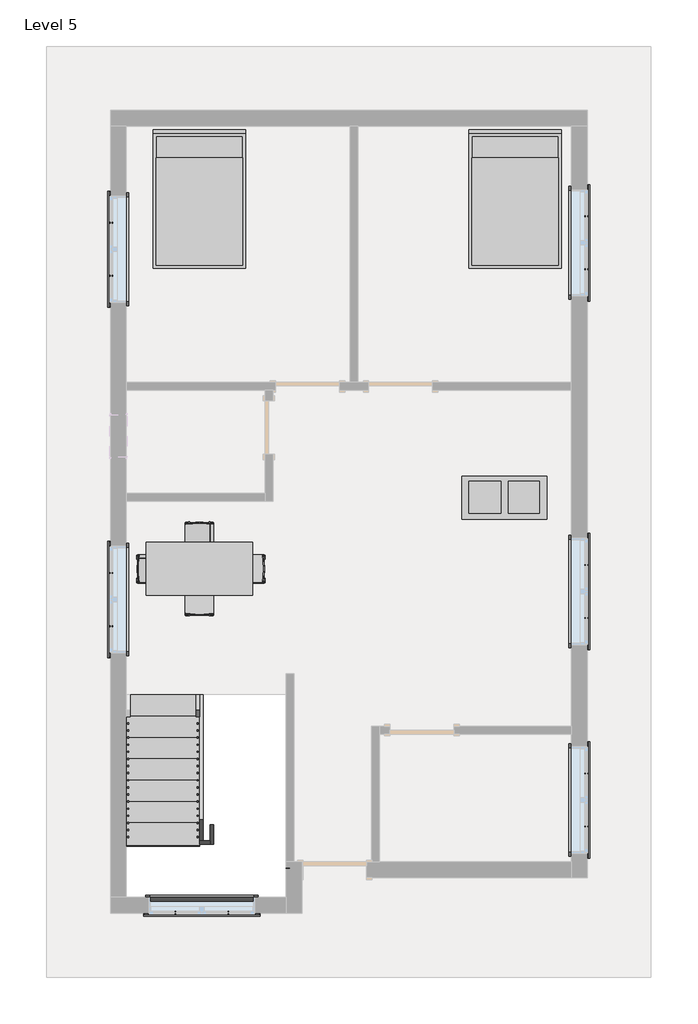
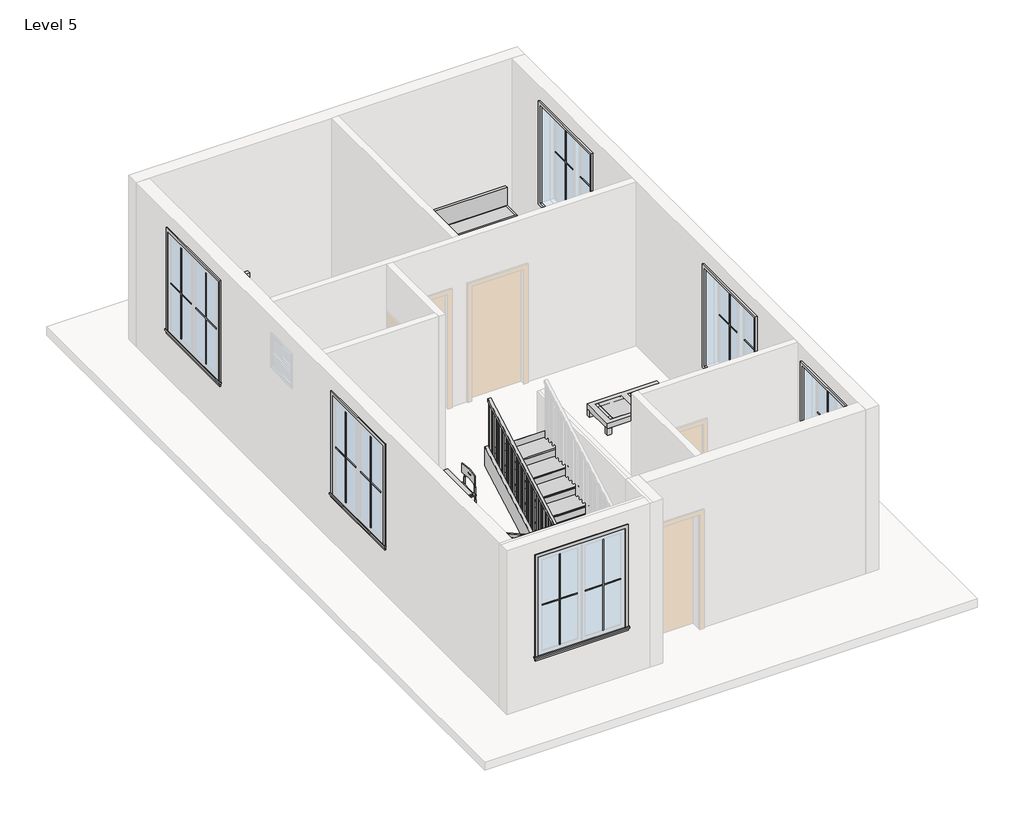
# One storey, part 3 of 3: 25 proxies, 6 members, 3 furniture elements, 1 railing, 1 stair flight.
"""IFC4 building model written with IfcOpenShell, lengths in millimetres."""

from ifc_helpers import new_model, si_unit, frame, origin, place, context, project, spatial, polyline, outline, extrude, faceted_brep, transform, mapped, element, save
from components import muntin_pattern_2x2_muntin_pattern_2x2_f6a80940, muntin_pattern_2x2_muntin_pattern_2x2_09b00a1c, trim_window_exterior_flat_with_sill_698ed857, trim_window_interior_flat_picture_frame_92551a5e, coffee_table_with_brass_mullions_11320_coffee_table_with_5962bef7, bed_17739_bed_17739_15c61121, dining_table_w_chairs_11374_0cdfc61b, stair_flight_bd25c6f5

model = new_model("IFC4")

# Units and contexts
model_context = context("Model", 3, world=origin())
ifc_project = project(units=[si_unit("LENGTHUNIT", "METRE", prefix="MILLI")], contexts=[model_context])

# Site, building, storey
site = spatial("IfcSite", under=ifc_project)
building = spatial("IfcBuilding", under=site)
storey = spatial("IfcBuildingStorey", under=building, Name="Level 5", Elevation=12649.2)

# Proxies
placement = place(None, origin())
muntin_pattern_2x2_muntin_pattern_2x2_shape = muntin_pattern_2x2_muntin_pattern_2x2_f6a80940(model_context)
element("IfcBuildingElementProxy", 1, Name="Muntin Pattern_2x2 : Muntin Pattern_2x2", ObjectType="Muntin Pattern_2x2 : Muntin Pattern_2x2", at=placement, inside=storey, context=model_context, shape_type="MappedRepresentation", body=[
    mapped(muntin_pattern_2x2_muntin_pattern_2x2_shape, transform((-2773.368364, -6686.2830018, 13633.45), x_axis=(-1.0, 0.0, 0.0), y_axis=(0.0, -1.0, 0.0), z_axis=(0.0, 0.0, 1.0))),
])
element("IfcBuildingElementProxy", 2, Name="Muntin Pattern_2x2 : Muntin Pattern_2x2", ObjectType="Muntin Pattern_2x2 : Muntin Pattern_2x2", at=placement, inside=storey, context=model_context, shape_type="MappedRepresentation", body=[
    mapped(muntin_pattern_2x2_muntin_pattern_2x2_shape, transform((2349.494136, -4693.9705018, 13633.45), x_axis=(0.0, -1.0, 0.0), y_axis=(1.0, 0.0, 0.0), z_axis=(0.0, 0.0, 1.0))),
])
element("IfcBuildingElementProxy", 3, Name="Muntin Pattern_2x2 : Muntin Pattern_2x2", ObjectType="Muntin Pattern_2x2 : Muntin Pattern_2x2", at=placement, inside=storey, context=model_context, shape_type="MappedRepresentation", body=[
    mapped(muntin_pattern_2x2_muntin_pattern_2x2_shape, transform((2349.494136, -1712.6455018, 13633.45), x_axis=(0.0, -1.0, 0.0), y_axis=(1.0, 0.0, 0.0), z_axis=(0.0, 0.0, 1.0))),
])
element("IfcBuildingElementProxy", 4, Name="Muntin Pattern_2x2 : Muntin Pattern_2x2", ObjectType="Muntin Pattern_2x2 : Muntin Pattern_2x2", at=placement, inside=storey, context=model_context, shape_type="MappedRepresentation", body=[
    mapped(muntin_pattern_2x2_muntin_pattern_2x2_shape, transform((-4451.355864, -2586.5525081, 13633.45), x_axis=(0.0, 1.0, 0.0), y_axis=(-1.0, 0.0, 0.0), z_axis=(0.0, 0.0, 1.0))),
])
element("IfcBuildingElementProxy", 5, Name="Muntin Pattern_2x2 : Muntin Pattern_2x2", ObjectType="Muntin Pattern_2x2 : Muntin Pattern_2x2", at=placement, inside=storey, context=model_context, shape_type="MappedRepresentation", body=[
    mapped(muntin_pattern_2x2_muntin_pattern_2x2_shape, transform((2349.494136, 3272.1044982, 13633.45), x_axis=(0.0, -1.0, 0.0), y_axis=(1.0, 0.0, 0.0), z_axis=(0.0, 0.0, 1.0))),
])
element("IfcBuildingElementProxy", 6, Name="Muntin Pattern_2x2 : Muntin Pattern_2x2", ObjectType="Muntin Pattern_2x2 : Muntin Pattern_2x2", at=placement, inside=storey, context=model_context, shape_type="MappedRepresentation", body=[
    mapped(muntin_pattern_2x2_muntin_pattern_2x2_shape, transform((-4451.355864, 2421.2162133, 13633.45), x_axis=(0.0, 1.0, 0.0), y_axis=(-1.0, 0.0, 0.0), z_axis=(0.0, 0.0, 1.0))),
])
muntin_pattern_2x2_muntin_pattern_2x2_2_shape = muntin_pattern_2x2_muntin_pattern_2x2_09b00a1c(model_context)
element("IfcBuildingElementProxy", 7, Name="Muntin Pattern_2x2 : Muntin Pattern_2x2", ObjectType="Muntin Pattern_2x2 : Muntin Pattern_2x2", at=placement, inside=storey, context=model_context, shape_type="MappedRepresentation", body=[
    mapped(muntin_pattern_2x2_muntin_pattern_2x2_2_shape, transform((-3532.193364, -6686.2830018, 13633.45), x_axis=(1.0, 0.0, 0.0), y_axis=(0.0, 1.0, 0.0), z_axis=(0.0, 0.0, 1.0))),
])
element("IfcBuildingElementProxy", 8, Name="Muntin Pattern_2x2 : Muntin Pattern_2x2", ObjectType="Muntin Pattern_2x2 : Muntin Pattern_2x2", at=placement, inside=storey, context=model_context, shape_type="MappedRepresentation", body=[
    mapped(muntin_pattern_2x2_muntin_pattern_2x2_2_shape, transform((2349.494136, -5452.7955018, 13633.45), x_axis=(0.0, 1.0, 0.0), y_axis=(-1.0, 0.0, 0.0), z_axis=(0.0, 0.0, 1.0))),
])
element("IfcBuildingElementProxy", 9, Name="Muntin Pattern_2x2 : Muntin Pattern_2x2", ObjectType="Muntin Pattern_2x2 : Muntin Pattern_2x2", at=placement, inside=storey, context=model_context, shape_type="MappedRepresentation", body=[
    mapped(muntin_pattern_2x2_muntin_pattern_2x2_2_shape, transform((2349.494136, -2471.4705018, 13633.45), x_axis=(0.0, 1.0, 0.0), y_axis=(-1.0, 0.0, 0.0), z_axis=(0.0, 0.0, 1.0))),
])
element("IfcBuildingElementProxy", 10, Name="Muntin Pattern_2x2 : Muntin Pattern_2x2", ObjectType="Muntin Pattern_2x2 : Muntin Pattern_2x2", at=placement, inside=storey, context=model_context, shape_type="MappedRepresentation", body=[
    mapped(muntin_pattern_2x2_muntin_pattern_2x2_2_shape, transform((-4451.355864, -1827.7275081, 13633.45), x_axis=(0.0, -1.0, 0.0), y_axis=(1.0, 0.0, 0.0), z_axis=(0.0, 0.0, 1.0))),
])
element("IfcBuildingElementProxy", 11, Name="Muntin Pattern_2x2 : Muntin Pattern_2x2", ObjectType="Muntin Pattern_2x2 : Muntin Pattern_2x2", at=placement, inside=storey, context=model_context, shape_type="MappedRepresentation", body=[
    mapped(muntin_pattern_2x2_muntin_pattern_2x2_2_shape, transform((2349.494136, 2513.2794982, 13633.45), x_axis=(0.0, 1.0, 0.0), y_axis=(-1.0, 0.0, 0.0), z_axis=(0.0, 0.0, 1.0))),
])
element("IfcBuildingElementProxy", 12, Name="Muntin Pattern_2x2 : Muntin Pattern_2x2", ObjectType="Muntin Pattern_2x2 : Muntin Pattern_2x2", at=placement, inside=storey, context=model_context, shape_type="MappedRepresentation", body=[
    mapped(muntin_pattern_2x2_muntin_pattern_2x2_2_shape, transform((-4451.355864, 3180.0412133, 13633.45), x_axis=(0.0, -1.0, 0.0), y_axis=(1.0, 0.0, 0.0), z_axis=(0.0, 0.0, 1.0))),
])
trim_window_exterior_flat_with_sill_shape = trim_window_exterior_flat_with_sill_698ed857(model_context)
element("IfcBuildingElementProxy", 13, Name="Trim-Window-Exterior-Flat : with Sill", ObjectType="Trim-Window-Exterior-Flat : with Sill", at=placement, inside=storey, context=model_context, shape_type="MappedRepresentation", body=[
    mapped(trim_window_exterior_flat_with_sill_shape, transform((-3152.780864, -6695.8080018, 15392.4), x_axis=(1.0, 0.0, 0.0), y_axis=(0.0, 0.0, 1.0), z_axis=(0.0, -1.0, 0.0))),
])
element("IfcBuildingElementProxy", 14, Name="Trim-Window-Exterior-Flat : with Sill", ObjectType="Trim-Window-Exterior-Flat : with Sill", at=placement, inside=storey, context=model_context, shape_type="MappedRepresentation", body=[
    mapped(trim_window_exterior_flat_with_sill_shape, transform((2359.019136, -5073.3830018, 15392.4), x_axis=(0.0, 1.0, 0.0), y_axis=(0.0, 0.0, 1.0), z_axis=(1.0, 0.0, 0.0))),
])
element("IfcBuildingElementProxy", 15, Name="Trim-Window-Exterior-Flat : with Sill", ObjectType="Trim-Window-Exterior-Flat : with Sill", at=placement, inside=storey, context=model_context, shape_type="MappedRepresentation", body=[
    mapped(trim_window_exterior_flat_with_sill_shape, transform((2359.019136, -2092.0580018, 15392.4), x_axis=(0.0, 1.0, 0.0), y_axis=(0.0, 0.0, 1.0), z_axis=(1.0, 0.0, 0.0))),
])
element("IfcBuildingElementProxy", 16, Name="Trim-Window-Exterior-Flat : with Sill", ObjectType="Trim-Window-Exterior-Flat : with Sill", at=placement, inside=storey, context=model_context, shape_type="MappedRepresentation", body=[
    mapped(trim_window_exterior_flat_with_sill_shape, transform((-4460.880864, -2207.1400081, 15392.4), x_axis=(0.0, -1.0, 0.0), y_axis=(0.0, 0.0, 1.0), z_axis=(-1.0, 0.0, 0.0))),
])
element("IfcBuildingElementProxy", 17, Name="Trim-Window-Exterior-Flat : with Sill", ObjectType="Trim-Window-Exterior-Flat : with Sill", at=placement, inside=storey, context=model_context, shape_type="MappedRepresentation", body=[
    mapped(trim_window_exterior_flat_with_sill_shape, transform((2359.019136, 2892.6919982, 15392.4), x_axis=(0.0, 1.0, 0.0), y_axis=(0.0, 0.0, 1.0), z_axis=(1.0, 0.0, 0.0))),
])
element("IfcBuildingElementProxy", 18, Name="Trim-Window-Exterior-Flat : with Sill", ObjectType="Trim-Window-Exterior-Flat : with Sill", at=placement, inside=storey, context=model_context, shape_type="MappedRepresentation", body=[
    mapped(trim_window_exterior_flat_with_sill_shape, transform((-4460.880864, 2800.6287133, 15392.4), x_axis=(0.0, -1.0, 0.0), y_axis=(0.0, 0.0, 1.0), z_axis=(-1.0, 0.0, 0.0))),
])
trim_window_interior_flat_picture_frame_shape = trim_window_interior_flat_picture_frame_92551a5e(model_context)
element("IfcBuildingElementProxy", 19, Name="Trim-Window-Interior-Flat : Picture Frame", ObjectType="Trim-Window-Interior-Flat : Picture Frame", at=placement, inside=storey, context=model_context, shape_type="MappedRepresentation", body=[
    mapped(trim_window_interior_flat_picture_frame_shape, transform((-3152.780864, -6467.2080018, 15392.4), x_axis=(-1.0, 0.0, 0.0), y_axis=(0.0, 0.0, 1.0), z_axis=(0.0, 1.0, 0.0))),
])
element("IfcBuildingElementProxy", 20, Name="Trim-Window-Interior-Flat : Picture Frame", ObjectType="Trim-Window-Interior-Flat : Picture Frame", at=placement, inside=storey, context=model_context, shape_type="MappedRepresentation", body=[
    mapped(trim_window_interior_flat_picture_frame_shape, transform((2130.419136, -5073.3830018, 15392.4), x_axis=(0.0, -1.0, 0.0), y_axis=(0.0, 0.0, 1.0), z_axis=(-1.0, 0.0, 0.0))),
])
element("IfcBuildingElementProxy", 21, Name="Trim-Window-Interior-Flat : Picture Frame", ObjectType="Trim-Window-Interior-Flat : Picture Frame", at=placement, inside=storey, context=model_context, shape_type="MappedRepresentation", body=[
    mapped(trim_window_interior_flat_picture_frame_shape, transform((2130.419136, -2092.0580018, 15392.4), x_axis=(0.0, -1.0, 0.0), y_axis=(0.0, 0.0, 1.0), z_axis=(-1.0, 0.0, 0.0))),
])
element("IfcBuildingElementProxy", 22, Name="Trim-Window-Interior-Flat : Picture Frame", ObjectType="Trim-Window-Interior-Flat : Picture Frame", at=placement, inside=storey, context=model_context, shape_type="MappedRepresentation", body=[
    mapped(trim_window_interior_flat_picture_frame_shape, transform((-4232.280864, -2207.1400081, 15392.4), x_axis=(0.0, 1.0, 0.0), y_axis=(0.0, 0.0, 1.0), z_axis=(1.0, 0.0, 0.0))),
])
element("IfcBuildingElementProxy", 23, Name="Trim-Window-Interior-Flat : Picture Frame", ObjectType="Trim-Window-Interior-Flat : Picture Frame", at=placement, inside=storey, context=model_context, shape_type="MappedRepresentation", body=[
    mapped(trim_window_interior_flat_picture_frame_shape, transform((2130.419136, 2892.6919982, 15392.4), x_axis=(0.0, -1.0, 0.0), y_axis=(0.0, 0.0, 1.0), z_axis=(-1.0, 0.0, 0.0))),
])
element("IfcBuildingElementProxy", 24, Name="Trim-Window-Interior-Flat : Picture Frame", ObjectType="Trim-Window-Interior-Flat : Picture Frame", at=placement, inside=storey, context=model_context, shape_type="MappedRepresentation", body=[
    mapped(trim_window_interior_flat_picture_frame_shape, transform((-4232.280864, 2800.6287133, 15392.4), x_axis=(0.0, 1.0, 0.0), y_axis=(0.0, 0.0, 1.0), z_axis=(1.0, 0.0, 0.0))),
])
coffee_table_with_brass_mullions_11320_coffee_table_with_shape = coffee_table_with_brass_mullions_11320_coffee_table_with_5962bef7(model_context)
element("IfcBuildingElementProxy", 25, Name="coffee_table_with_brass_mullions_11320 : coffee_table_with_brass_mullions_11320", ObjectType="coffee_table_with_brass_mullions_11320 : coffee_table_with_brass_mullions_11320", at=placement, inside=storey, context=model_context, shape_type="MappedRepresentation", body=[
    mapped(coffee_table_with_brass_mullions_11320_coffee_table_with_shape, transform((1812.3816081, -1181.1001099, 12649.2), x_axis=(1.0, 0.0, 0.0), y_axis=(0.0, 1.0, 0.0), z_axis=(0.0, 0.0, 1.0))),
])

# Furniture
bed_17739_bed_17739_shape = bed_17739_bed_17739_15c61121(model_context)
element("IfcFurniture", 26, ObjectType="Bed_17739 : Bed_17739", at=placement, inside=storey, context=model_context, shape_type="MappedRepresentation", body=[
    mapped(bed_17739_bed_17739_shape, transform((1328.5116081, 3496.3098901, 12649.2), x_axis=(1.0, 0.0, 0.0), y_axis=(0.0, 1.0, 0.0), z_axis=(0.0, 0.0, 1.0))),
])
element("IfcFurniture", 27, ObjectType="Bed_17739 : Bed_17739", at=placement, inside=storey, context=model_context, shape_type="MappedRepresentation", body=[
    mapped(bed_17739_bed_17739_shape, transform((-3187.6083919, 3496.3098901, 12649.2), x_axis=(1.0, 0.0, 0.0), y_axis=(0.0, 1.0, 0.0), z_axis=(0.0, 0.0, 1.0))),
])
dining_table_w_chairs_11374_shape = dining_table_w_chairs_11374_0cdfc61b(model_context)
element("IfcFurniture", 28, ObjectType="Dining_Table_w_Chairs_11374", at=placement, inside=storey, context=model_context, shape_type="MappedRepresentation", body=[
    mapped(dining_table_w_chairs_11374_shape, transform((-3205.8741586, -1863.0511877, 12649.2), x_axis=(1.0, 0.0, 0.0), y_axis=(0.0, 1.0, 0.0), z_axis=(0.0, 0.0, 1.0))),
])

# Members
element("IfcMember", 29, ObjectType="Stringer - 2\" Width", at=placement, inside=storey, context=model_context, shape_type="SweptSolid", body=[
    extrude(outline(polyline([(-3571.6080018, 12856.7983948), (-3571.6080018, 12649.2), (-3825.5525046, 12649.2), (-5654.4080018, 13665.2308318), (-5654.4080018, 14013.9095059), (-3571.6080018, 12856.7983948)])), frame((-3187.6083919, 0.0, 0.0), z_axis=(1.0, 0.0, 0.0), x_axis=(0.0, 1.0, 0.0)), (0.0, 0.0, 1.0), 50.8),
])
element("IfcMember", 30, ObjectType="Stringer - 2\" Width", at=placement, inside=storey, context=model_context, shape_type="SweptSolid", body=[
    extrude(outline(polyline([(-3187.6083919, -5705.2080018), (-3187.6083919, -5654.4080018), (-3035.2083919, -5654.4080018), (-3035.2083919, -5705.2080018), (-3187.6083919, -5705.2080018)])), frame((0.0, 0.0, 13775.2666667), z_axis=(0.0, 0.0, 1.0), x_axis=(1.0, 0.0, 0.0)), (0.0, 0.0, 1.0), 304.8),
])
element("IfcMember", 31, ObjectType="Stringer - 2\" Width", at=placement, inside=storey, context=model_context, shape_type="SweptSolid", body=[
    extrude(outline(polyline([(-5705.2080018, 13775.2666667), (-5705.2080018, 14042.1317281), (-3571.6080018, 15227.4650614), (-3571.6080018, 14878.7863873), (-5557.943499, 13775.2666667), (-5705.2080018, 13775.2666667)])), frame((-3035.2083919, 0.0, 0.0), z_axis=(1.0, 0.0, 0.0), x_axis=(0.0, 1.0, 0.0)), (0.0, 0.0, 1.0), 50.8),
])
element("IfcMember", 32, ObjectType="Stringer - 2\" Width", at=placement, inside=storey, context=model_context, shape_type="SweptSolid", body=[
    extrude(outline(polyline([(-3571.6080018, 12856.7983948), (-3571.6080018, 12649.2), (-3825.5525046, 12649.2), (-6401.1125046, 14080.0666667), (-5773.4908912, 14080.0666667), (-3571.6080018, 12856.7983948)])), frame((-4283.080864, 0.0, 0.0), z_axis=(1.0, 0.0, 0.0), x_axis=(0.0, 1.0, 0.0)), (0.0, 0.0, 1.0), 50.8),
])
element("IfcMember", 33, ObjectType="Stringer - 2\" Width", at=placement, inside=storey, context=model_context, shape_type="SweptSolid", body=[
    extrude(outline(polyline([(-4283.080864, -6518.0080018), (-4283.080864, -6467.2080018), (-1946.280864, -6467.2080018), (-1946.280864, -6518.0080018), (-4283.080864, -6518.0080018)])), frame((0.0, 0.0, 13775.2666667), z_axis=(0.0, 0.0, 1.0), x_axis=(1.0, 0.0, 0.0)), (0.0, 0.0, 1.0), 304.8),
])
element("IfcMember", 34, ObjectType="Stringer - 2\" Width", at=placement, inside=storey, context=model_context, shape_type="SweptSolid", body=[
    extrude(outline(polyline([(-6185.5651124, 13775.2666667), (-3571.6080018, 15227.4650614), (-3571.6080018, 14878.7863873), (-5557.943499, 13775.2666667), (-6185.5651124, 13775.2666667)])), frame((-1946.280864, 0.0, 0.0), z_axis=(1.0, 0.0, 0.0), x_axis=(0.0, 1.0, 0.0)), (0.0, 0.0, 1.0), 50.8),
])

# Railing
element("IfcRailing", 35, ObjectType="Handrail - Rectangular", at=placement, inside=storey, context=model_context, shape_type="SolidModel", body=[
    faceted_brep([(-3187.6083919, -3571.6080018, 13732.9333333), (-3187.6083919, -3571.6080018, 13674.820221), (-3238.4083919, -3571.6080018, 13674.820221), (-3238.4083919, -3571.6080018, 13732.9333333), (-3187.6083919, -5629.0080018, 14875.9333333), (-3187.6083919, -5679.8080018, 14846.0424432), (-3238.4083919, -5679.8080018, 14846.0424432), (-3238.4083919, -5629.0080018, 14875.9333333), (-3187.6083919, -5629.0080018, 14918.2666667), (-3187.6083919, -5679.8080018, 14867.4666667), (-3238.4083919, -5679.8080018, 14867.4666667), (-3238.4083919, -5629.0080018, 14918.2666667), (-3187.6083919, -5705.2080018, 14918.2666667), (-3187.6083919, -5705.2080018, 14867.4666667), (-3238.4083919, -5756.0080018, 14867.4666667), (-3238.4083919, -5756.0080018, 14918.2666667), (-3111.4083919, -5705.2080018, 14918.2666667), (-3111.4083919, -5705.2080018, 14867.4666667), (-3111.4083919, -5756.0080018, 14867.4666667), (-3111.4083919, -5756.0080018, 14918.2666667), (-3060.6083919, -5705.2080018, 14918.2666667), (-3009.8083919, -5705.2080018, 14867.4666667), (-3009.8083919, -5756.0080018, 14867.4666667), (-3060.6083919, -5756.0080018, 14918.2666667), (-3060.6083919, -5705.2080018, 14960.6), (-3009.8083919, -5705.2080018, 14909.8), (-3009.8083919, -5756.0080018, 14909.8), (-3060.6083919, -5756.0080018, 14960.6), (-2984.4083919, -5705.2080018, 14960.6), (-2984.4083919, -5705.2080018, 14909.8), (-2933.6083919, -5756.0080018, 14909.8), (-2933.6083919, -5756.0080018, 14960.6), (-2984.4083919, -5629.0080018, 14960.6), (-2984.4083919, -5615.8443995, 14909.8), (-2933.6083919, -5615.8443995, 14909.8), (-2933.6083919, -5629.0080018, 14960.6), (-2984.4083919, -3571.6080018, 16103.6), (-2933.6083919, -3571.6080018, 16103.6), (-2933.6083919, -3571.6080018, 16045.4868876), (-2984.4083919, -3571.6080018, 16045.4868876)], [[[0, 1, 2, 3]], [[1, 0, 4, 5]], [[2, 1, 5, 6]], [[3, 2, 6, 7]], [[0, 3, 7, 4]], [[5, 4, 8, 9]], [[6, 5, 9, 10]], [[7, 6, 10, 11]], [[4, 7, 11, 8]], [[9, 8, 12, 13]], [[10, 9, 13, 14]], [[11, 10, 14, 15]], [[8, 11, 15, 12]], [[13, 12, 16, 17]], [[14, 13, 17, 18]], [[15, 14, 18, 19]], [[12, 15, 19, 16]], [[17, 16, 20, 21]], [[18, 17, 21, 22]], [[19, 18, 22, 23]], [[16, 19, 23, 20]], [[21, 20, 24, 25]], [[22, 21, 25, 26]], [[23, 22, 26, 27]], [[20, 23, 27, 24]], [[25, 24, 28, 29]], [[26, 25, 29, 30]], [[27, 26, 30, 31]], [[24, 27, 31, 28]], [[29, 28, 32, 33]], [[30, 29, 33, 34]], [[31, 30, 34, 35]], [[28, 31, 35, 32]], [[36, 37, 38, 39]], [[33, 32, 36, 39]], [[34, 33, 39, 38]], [[35, 34, 38, 37]], [[32, 35, 37, 36]]]),
    extrude(outline(polyline([(-3587.4830018, 16036.6674432), (-3587.4830018, 15019.8666667), (-3606.5330018, 15019.8666667), (-3606.5330018, 16026.0841099), (-3587.4830018, 16036.6674432)])), frame((-2968.5333919, 0.0, 0.0), z_axis=(1.0, 0.0, 0.0), x_axis=(0.0, 1.0, 0.0)), (0.0, 0.0, 1.0), 19.05),
    extrude(outline(polyline([(-3689.0830018, 15980.2229988), (-3689.0830018, 15019.8666667), (-3708.1330018, 15019.8666667), (-3708.1330018, 15969.6396654), (-3689.0830018, 15980.2229988)])), frame((-2968.5333919, 0.0, 0.0), z_axis=(1.0, 0.0, 0.0), x_axis=(0.0, 1.0, 0.0)), (0.0, 0.0, 1.0), 19.05),
    extrude(outline(polyline([(-3790.6830018, 15923.7785543), (-3790.6830018, 15019.8666667), (-3809.7330018, 15019.8666667), (-3809.7330018, 15913.195221), (-3790.6830018, 15923.7785543)])), frame((-2968.5333919, 0.0, 0.0), z_axis=(1.0, 0.0, 0.0), x_axis=(0.0, 1.0, 0.0)), (0.0, 0.0, 1.0), 19.05),
    extrude(outline(polyline([(-3892.2830018, 15867.3341099), (-3892.2830018, 14850.5333333), (-3911.3330018, 14850.5333333), (-3911.3330018, 15856.7507765), (-3892.2830018, 15867.3341099)])), frame((-2968.5333919, 0.0, 0.0), z_axis=(1.0, 0.0, 0.0), x_axis=(0.0, 1.0, 0.0)), (0.0, 0.0, 1.0), 19.05),
    extrude(outline(polyline([(-3993.8830018, 15810.8896654), (-3993.8830018, 14850.5333333), (-4012.9330018, 14850.5333333), (-4012.9330018, 15800.3063321), (-3993.8830018, 15810.8896654)])), frame((-2968.5333919, 0.0, 0.0), z_axis=(1.0, 0.0, 0.0), x_axis=(0.0, 1.0, 0.0)), (0.0, 0.0, 1.0), 19.05),
    extrude(outline(polyline([(-4095.4830018, 15754.445221), (-4095.4830018, 14850.5333333), (-4114.5330018, 14850.5333333), (-4114.5330018, 15743.8618876), (-4095.4830018, 15754.445221)])), frame((-2968.5333919, 0.0, 0.0), z_axis=(1.0, 0.0, 0.0), x_axis=(0.0, 1.0, 0.0)), (0.0, 0.0, 1.0), 19.05),
    extrude(outline(polyline([(-4197.0830018, 15698.0007765), (-4197.0830018, 14681.2), (-4216.1330018, 14681.2), (-4216.1330018, 15687.4174432), (-4197.0830018, 15698.0007765)])), frame((-2968.5333919, 0.0, 0.0), z_axis=(1.0, 0.0, 0.0), x_axis=(0.0, 1.0, 0.0)), (0.0, 0.0, 1.0), 19.05),
    extrude(outline(polyline([(-4298.6830018, 15641.5563321), (-4298.6830018, 14681.2), (-4317.7330018, 14681.2), (-4317.7330018, 15630.9729988), (-4298.6830018, 15641.5563321)])), frame((-2968.5333919, 0.0, 0.0), z_axis=(1.0, 0.0, 0.0), x_axis=(0.0, 1.0, 0.0)), (0.0, 0.0, 1.0), 19.05),
    extrude(outline(polyline([(-4400.2830018, 15585.1118876), (-4400.2830018, 14681.2), (-4419.3330018, 14681.2), (-4419.3330018, 15574.5285543), (-4400.2830018, 15585.1118876)])), frame((-2968.5333919, 0.0, 0.0), z_axis=(1.0, 0.0, 0.0), x_axis=(0.0, 1.0, 0.0)), (0.0, 0.0, 1.0), 19.05),
    extrude(outline(polyline([(-4501.8830018, 15528.6674432), (-4501.8830018, 14511.8666667), (-4520.9330018, 14511.8666667), (-4520.9330018, 15518.0841099), (-4501.8830018, 15528.6674432)])), frame((-2968.5333919, 0.0, 0.0), z_axis=(1.0, 0.0, 0.0), x_axis=(0.0, 1.0, 0.0)), (0.0, 0.0, 1.0), 19.05),
    extrude(outline(polyline([(-4603.4830018, 15472.2229988), (-4603.4830018, 14511.8666667), (-4622.5330018, 14511.8666667), (-4622.5330018, 15461.6396654), (-4603.4830018, 15472.2229988)])), frame((-2968.5333919, 0.0, 0.0), z_axis=(1.0, 0.0, 0.0), x_axis=(0.0, 1.0, 0.0)), (0.0, 0.0, 1.0), 19.05),
    extrude(outline(polyline([(-4705.0830018, 15415.7785543), (-4705.0830018, 14511.8666667), (-4724.1330018, 14511.8666667), (-4724.1330018, 15405.195221), (-4705.0830018, 15415.7785543)])), frame((-2968.5333919, 0.0, 0.0), z_axis=(1.0, 0.0, 0.0), x_axis=(0.0, 1.0, 0.0)), (0.0, 0.0, 1.0), 19.05),
    extrude(outline(polyline([(-4806.6830018, 15359.3341099), (-4806.6830018, 14342.5333333), (-4825.7330018, 14342.5333333), (-4825.7330018, 15348.7507765), (-4806.6830018, 15359.3341099)])), frame((-2968.5333919, 0.0, 0.0), z_axis=(1.0, 0.0, 0.0), x_axis=(0.0, 1.0, 0.0)), (0.0, 0.0, 1.0), 19.05),
    extrude(outline(polyline([(-4908.2830018, 15302.8896654), (-4908.2830018, 14342.5333333), (-4927.3330018, 14342.5333333), (-4927.3330018, 15292.3063321), (-4908.2830018, 15302.8896654)])), frame((-2968.5333919, 0.0, 0.0), z_axis=(1.0, 0.0, 0.0), x_axis=(0.0, 1.0, 0.0)), (0.0, 0.0, 1.0), 19.05),
    extrude(outline(polyline([(-5009.8830018, 15246.445221), (-5009.8830018, 14342.5333333), (-5028.9330018, 14342.5333333), (-5028.9330018, 15235.8618876), (-5009.8830018, 15246.445221)])), frame((-2968.5333919, 0.0, 0.0), z_axis=(1.0, 0.0, 0.0), x_axis=(0.0, 1.0, 0.0)), (0.0, 0.0, 1.0), 19.05),
    extrude(outline(polyline([(-5111.4830018, 15190.0007765), (-5111.4830018, 14173.2), (-5130.5330018, 14173.2), (-5130.5330018, 15179.4174432), (-5111.4830018, 15190.0007765)])), frame((-2968.5333919, 0.0, 0.0), z_axis=(1.0, 0.0, 0.0), x_axis=(0.0, 1.0, 0.0)), (0.0, 0.0, 1.0), 19.05),
    extrude(outline(polyline([(-5213.0830018, 15133.5563321), (-5213.0830018, 14173.2), (-5232.1330018, 14173.2), (-5232.1330018, 15122.9729988), (-5213.0830018, 15133.5563321)])), frame((-2968.5333919, 0.0, 0.0), z_axis=(1.0, 0.0, 0.0), x_axis=(0.0, 1.0, 0.0)), (0.0, 0.0, 1.0), 19.05),
    extrude(outline(polyline([(-5314.6830018, 15077.1118876), (-5314.6830018, 14173.2), (-5333.7330018, 14173.2), (-5333.7330018, 15066.5285543), (-5314.6830018, 15077.1118876)])), frame((-2968.5333919, 0.0, 0.0), z_axis=(1.0, 0.0, 0.0), x_axis=(0.0, 1.0, 0.0)), (0.0, 0.0, 1.0), 19.05),
    extrude(outline(polyline([(-5416.2830018, 15020.6674432), (-5416.2830018, 14003.8666667), (-5435.3330018, 14003.8666667), (-5435.3330018, 15010.0841099), (-5416.2830018, 15020.6674432)])), frame((-2968.5333919, 0.0, 0.0), z_axis=(1.0, 0.0, 0.0), x_axis=(0.0, 1.0, 0.0)), (0.0, 0.0, 1.0), 19.05),
    extrude(outline(polyline([(-5517.8830018, 14964.2229988), (-5517.8830018, 14003.8666667), (-5536.9330018, 14003.8666667), (-5536.9330018, 14953.6396654), (-5517.8830018, 14964.2229988)])), frame((-2968.5333919, 0.0, 0.0), z_axis=(1.0, 0.0, 0.0), x_axis=(0.0, 1.0, 0.0)), (0.0, 0.0, 1.0), 19.05),
    extrude(outline(polyline([(-5619.4830018, 14907.7785543), (-5619.4830018, 14003.8666667), (-5638.5330018, 14003.8666667), (-5638.5330018, 14897.195221), (-5619.4830018, 14907.7785543)])), frame((-2968.5333919, 0.0, 0.0), z_axis=(1.0, 0.0, 0.0), x_axis=(0.0, 1.0, 0.0)), (0.0, 0.0, 1.0), 19.05),
    extrude(outline(polyline([(-3019.3333919, -5721.0830018), (-3000.2833919, -5721.0830018), (-3000.2833919, -5740.1330018), (-3019.3333919, -5740.1330018), (-3019.3333919, -5721.0830018)])), frame((0.0, 0.0, 14003.8666667), z_axis=(0.0, 0.0, 1.0), x_axis=(1.0, 0.0, 0.0)), (0.0, 0.0, 1.0), 905.9333333),
    extrude(outline(polyline([(-3120.9333919, -5721.0830018), (-3101.8833919, -5721.0830018), (-3101.8833919, -5740.1330018), (-3120.9333919, -5740.1330018), (-3120.9333919, -5721.0830018)])), frame((0.0, 0.0, 14003.8666667), z_axis=(0.0, 0.0, 1.0), x_axis=(1.0, 0.0, 0.0)), (0.0, 0.0, 1.0), 863.6),
    extrude(outline(polyline([(-3203.4833919, -5695.6830018), (-3203.4833919, -5714.7330018), (-3222.5333919, -5714.7330018), (-3222.5333919, -5695.6830018), (-3203.4833919, -5695.6830018)])), frame((0.0, 0.0, 14003.8666667), z_axis=(0.0, 0.0, 1.0), x_axis=(1.0, 0.0, 0.0)), (0.0, 0.0, 1.0), 863.6),
    extrude(outline(polyline([(-5594.0830018, 14798.4174432), (-5594.0830018, 13834.5333333), (-5613.1330018, 13834.5333333), (-5613.1330018, 14809.0007765), (-5594.0830018, 14798.4174432)])), frame((-3222.5333919, 0.0, 0.0), z_axis=(1.0, 0.0, 0.0), x_axis=(0.0, 1.0, 0.0)), (0.0, 0.0, 1.0), 19.05),
    extrude(outline(polyline([(-5492.4830018, 14741.9729988), (-5492.4830018, 13834.5333333), (-5511.5330018, 13834.5333333), (-5511.5330018, 14752.5563321), (-5492.4830018, 14741.9729988)])), frame((-3222.5333919, 0.0, 0.0), z_axis=(1.0, 0.0, 0.0), x_axis=(0.0, 1.0, 0.0)), (0.0, 0.0, 1.0), 19.05),
    extrude(outline(polyline([(-5390.8830018, 14685.5285543), (-5390.8830018, 13834.5333333), (-5409.9330018, 13834.5333333), (-5409.9330018, 14696.1118876), (-5390.8830018, 14685.5285543)])), frame((-3222.5333919, 0.0, 0.0), z_axis=(1.0, 0.0, 0.0), x_axis=(0.0, 1.0, 0.0)), (0.0, 0.0, 1.0), 19.05),
    extrude(outline(polyline([(-5289.2830018, 14629.0841099), (-5289.2830018, 13665.2), (-5308.3330018, 13665.2), (-5308.3330018, 14639.6674432), (-5289.2830018, 14629.0841099)])), frame((-3222.5333919, 0.0, 0.0), z_axis=(1.0, 0.0, 0.0), x_axis=(0.0, 1.0, 0.0)), (0.0, 0.0, 1.0), 19.05),
    extrude(outline(polyline([(-5187.6830018, 14572.6396654), (-5187.6830018, 13665.2), (-5206.7330018, 13665.2), (-5206.7330018, 14583.2229988), (-5187.6830018, 14572.6396654)])), frame((-3222.5333919, 0.0, 0.0), z_axis=(1.0, 0.0, 0.0), x_axis=(0.0, 1.0, 0.0)), (0.0, 0.0, 1.0), 19.05),
    extrude(outline(polyline([(-5086.0830018, 14516.195221), (-5086.0830018, 13665.2), (-5105.1330018, 13665.2), (-5105.1330018, 14526.7785543), (-5086.0830018, 14516.195221)])), frame((-3222.5333919, 0.0, 0.0), z_axis=(1.0, 0.0, 0.0), x_axis=(0.0, 1.0, 0.0)), (0.0, 0.0, 1.0), 19.05),
    extrude(outline(polyline([(-4984.4830018, 14459.7507765), (-4984.4830018, 13495.8666667), (-5003.5330018, 13495.8666667), (-5003.5330018, 14470.3341099), (-4984.4830018, 14459.7507765)])), frame((-3222.5333919, 0.0, 0.0), z_axis=(1.0, 0.0, 0.0), x_axis=(0.0, 1.0, 0.0)), (0.0, 0.0, 1.0), 19.05),
    extrude(outline(polyline([(-4882.8830018, 14403.3063321), (-4882.8830018, 13495.8666667), (-4901.9330018, 13495.8666667), (-4901.9330018, 14413.8896654), (-4882.8830018, 14403.3063321)])), frame((-3222.5333919, 0.0, 0.0), z_axis=(1.0, 0.0, 0.0), x_axis=(0.0, 1.0, 0.0)), (0.0, 0.0, 1.0), 19.05),
    extrude(outline(polyline([(-4781.2830018, 14346.8618876), (-4781.2830018, 13495.8666667), (-4800.3330018, 13495.8666667), (-4800.3330018, 14357.445221), (-4781.2830018, 14346.8618876)])), frame((-3222.5333919, 0.0, 0.0), z_axis=(1.0, 0.0, 0.0), x_axis=(0.0, 1.0, 0.0)), (0.0, 0.0, 1.0), 19.05),
    extrude(outline(polyline([(-4679.6830018, 14290.4174432), (-4679.6830018, 13326.5333333), (-4698.7330018, 13326.5333333), (-4698.7330018, 14301.0007765), (-4679.6830018, 14290.4174432)])), frame((-3222.5333919, 0.0, 0.0), z_axis=(1.0, 0.0, 0.0), x_axis=(0.0, 1.0, 0.0)), (0.0, 0.0, 1.0), 19.05),
    extrude(outline(polyline([(-4578.0830018, 14233.9729988), (-4578.0830018, 13326.5333333), (-4597.1330018, 13326.5333333), (-4597.1330018, 14244.5563321), (-4578.0830018, 14233.9729988)])), frame((-3222.5333919, 0.0, 0.0), z_axis=(1.0, 0.0, 0.0), x_axis=(0.0, 1.0, 0.0)), (0.0, 0.0, 1.0), 19.05),
    extrude(outline(polyline([(-4476.4830018, 14177.5285543), (-4476.4830018, 13326.5333333), (-4495.5330018, 13326.5333333), (-4495.5330018, 14188.1118876), (-4476.4830018, 14177.5285543)])), frame((-3222.5333919, 0.0, 0.0), z_axis=(1.0, 0.0, 0.0), x_axis=(0.0, 1.0, 0.0)), (0.0, 0.0, 1.0), 19.05),
    extrude(outline(polyline([(-4374.8830018, 14121.0841099), (-4374.8830018, 13157.2), (-4393.9330018, 13157.2), (-4393.9330018, 14131.6674432), (-4374.8830018, 14121.0841099)])), frame((-3222.5333919, 0.0, 0.0), z_axis=(1.0, 0.0, 0.0), x_axis=(0.0, 1.0, 0.0)), (0.0, 0.0, 1.0), 19.05),
    extrude(outline(polyline([(-4273.2830018, 14064.6396654), (-4273.2830018, 13157.2), (-4292.3330018, 13157.2), (-4292.3330018, 14075.2229988), (-4273.2830018, 14064.6396654)])), frame((-3222.5333919, 0.0, 0.0), z_axis=(1.0, 0.0, 0.0), x_axis=(0.0, 1.0, 0.0)), (0.0, 0.0, 1.0), 19.05),
    extrude(outline(polyline([(-4171.6830018, 14008.195221), (-4171.6830018, 13157.2), (-4190.7330018, 13157.2), (-4190.7330018, 14018.7785543), (-4171.6830018, 14008.195221)])), frame((-3222.5333919, 0.0, 0.0), z_axis=(1.0, 0.0, 0.0), x_axis=(0.0, 1.0, 0.0)), (0.0, 0.0, 1.0), 19.05),
    extrude(outline(polyline([(-4070.0830018, 13951.7507765), (-4070.0830018, 12987.8666667), (-4089.1330018, 12987.8666667), (-4089.1330018, 13962.3341099), (-4070.0830018, 13951.7507765)])), frame((-3222.5333919, 0.0, 0.0), z_axis=(1.0, 0.0, 0.0), x_axis=(0.0, 1.0, 0.0)), (0.0, 0.0, 1.0), 19.05),
    extrude(outline(polyline([(-3968.4830018, 13895.3063321), (-3968.4830018, 12987.8666667), (-3987.5330018, 12987.8666667), (-3987.5330018, 13905.8896654), (-3968.4830018, 13895.3063321)])), frame((-3222.5333919, 0.0, 0.0), z_axis=(1.0, 0.0, 0.0), x_axis=(0.0, 1.0, 0.0)), (0.0, 0.0, 1.0), 19.05),
    extrude(outline(polyline([(-3866.8830018, 13838.8618876), (-3866.8830018, 12987.8666667), (-3885.9330018, 12987.8666667), (-3885.9330018, 13849.445221), (-3866.8830018, 13838.8618876)])), frame((-3222.5333919, 0.0, 0.0), z_axis=(1.0, 0.0, 0.0), x_axis=(0.0, 1.0, 0.0)), (0.0, 0.0, 1.0), 19.05),
    extrude(outline(polyline([(-3765.2830018, 13782.4174432), (-3765.2830018, 12818.5333333), (-3784.3330018, 12818.5333333), (-3784.3330018, 13793.0007765), (-3765.2830018, 13782.4174432)])), frame((-3222.5333919, 0.0, 0.0), z_axis=(1.0, 0.0, 0.0), x_axis=(0.0, 1.0, 0.0)), (0.0, 0.0, 1.0), 19.05),
    extrude(outline(polyline([(-3663.6830018, 13725.9729988), (-3663.6830018, 12818.5333333), (-3682.7330018, 12818.5333333), (-3682.7330018, 13736.5563321), (-3663.6830018, 13725.9729988)])), frame((-3222.5333919, 0.0, 0.0), z_axis=(1.0, 0.0, 0.0), x_axis=(0.0, 1.0, 0.0)), (0.0, 0.0, 1.0), 19.05),
    extrude(outline(polyline([(-2968.5333919, -5721.0830018), (-2949.4833919, -5721.0830018), (-2949.4833919, -5740.1330018), (-2968.5333919, -5740.1330018), (-2968.5333919, -5721.0830018)])), frame((0.0, 0.0, 14003.8666667), z_axis=(0.0, 0.0, 1.0), x_axis=(1.0, 0.0, 0.0)), (0.0, 0.0, 1.0), 905.9333333),
    extrude(outline(polyline([(-3203.4833919, -5721.0830018), (-3203.4833919, -5740.1330018), (-3222.5333919, -5740.1330018), (-3222.5333919, -5721.0830018), (-3203.4833919, -5721.0830018)])), frame((0.0, 0.0, 14003.8666667), z_axis=(0.0, 0.0, 1.0), x_axis=(1.0, 0.0, 0.0)), (0.0, 0.0, 1.0), 863.6),
    extrude(outline(polyline([(-3571.6080018, 16045.4868876), (-3571.6080018, 15019.8666667), (-3590.6580018, 15019.8666667), (-3590.6580018, 16034.9035543), (-3571.6080018, 16045.4868876)])), frame((-2968.5333919, 0.0, 0.0), z_axis=(1.0, 0.0, 0.0), x_axis=(0.0, 1.0, 0.0)), (0.0, 0.0, 1.0), 19.05),
    extrude(outline(polyline([(-3571.6080018, 13674.820221), (-3571.6080018, 12818.5333333), (-3590.6580018, 12818.5333333), (-3590.6580018, 13685.4035543), (-3571.6080018, 13674.820221)])), frame((-3222.5333919, 0.0, 0.0), z_axis=(1.0, 0.0, 0.0), x_axis=(0.0, 1.0, 0.0)), (0.0, 0.0, 1.0), 19.05),
])

# Stair flight
stair_flight_shape = stair_flight_bd25c6f5(model_context)
element("IfcStairFlight", 36, ObjectType="2\" Tread 1\" Nosing 1/4\" Riser", at=placement, inside=storey, context=model_context, shape_type="MappedRepresentation", body=[
    mapped(stair_flight_shape, transform((0.0, 0.0, 0.0), x_axis=(1.0, 0.0, 0.0), y_axis=(0.0, 1.0, 0.0), z_axis=(0.0, 0.0, 1.0))),
])

save(model, "model.ifc")

# Revit data of these elements
# Type "Muntin Pattern_2x2 : Muntin Pattern_2x2"
#   Width [instance default] = 4' - 0"
#   Thickness = 0' - 0 1/2"
#   Height [instance default] = 4' - 0"
#   Distance = 0' - 0 3/4"
#   Interior Material [instance default] = none
#   Exterior Material [instance default] = none
#   Default Elevation = 0
# Type "Trim-Window-Exterior-Flat : with Sill"
#   Trim Width = 0' - 2 1/4"
#   Trim Thickness_Picture Frame = 0' - 1 1/4"
#   Trim Thickness_with Sill = 0' - 0 3/4"
#   Sill Thickness = 0' - 1 1/4"
#   Opening Width [instance default] = 2' - 0"
#   Opening Height [instance default] = 3' - 0"
#   Default Elevation = 4' - 0"
#   Sill = yes
#   Picture Frame = no
#   Trim Material [instance default] = none
# Type "Trim-Window-Interior-Flat : Picture Frame"
#   Trim Thickness_Picture Frame = 0' - 1 1/4"
#   Trim Width = 0' - 2 1/4"
#   Trim Thickness_with Sill = 0' - 0 3/4"
#   Sill Thickness = 0' - 1 1/4"
#   Opening Width [instance default] = 2' - 0"
#   Opening Height [instance default] = 3' - 0"
#   Default Elevation = 4' - 0"
#   Sill = no
#   Picture Frame = yes
#   Trim Material [instance default] = none
# Type "coffee_table_with_brass_mullions_11320 : coffee_table_with_brass_mullions_11320"
#   Default Elevation = 0
# Type "Bed_17739 : Bed_17739"
#   Default Elevation = 0
# Type "Dining_Table_w_Chairs_11374"
#   Default Elevation = 0
#   Assembly Code = ""
# Type "Handrail - Rectangular"
#   Assembly Code = "C2010400"
#   built-in parameter 1008612 = 0.0416667 (stored number, unit not read)
#   built-in parameter 1008611 = 0.0416667 (stored number, unit not read)
#   built-in parameter 1008609 = 0.333333 (stored number, unit not read)
#   built-in parameter 1008604 = 0.166667 (stored number, unit not read)
#   built-in parameter 1008603 = 0.166667 (stored number, unit not read)
#   Railing Height = 3' - 0"
#   built-in parameter 1008630 = 2
#   built-in parameter 1008610 = 2
#   built-in parameter 1008618 = Baluster - Square : 3/4"
# Elements 1, 2, 3, 4, 5, 6, 7, 8, 9, 10, 11, 12 (IfcBuildingElementProxy, "Muntin Pattern_2x2 : Muntin Pattern_2x2")
#   Width = 2' - 0 5/8"
#   Height = 5' - 6 1/2"
#   Interior Material = Wood - Stained
#   Exterior Material = Clad - White
#   Phase Created = New Construction
#   Materials on its faces: "Clad - White", "Wood - Stained"
# Elements 13, 14, 15, 16, 17, 18 (IfcBuildingElementProxy, "Trim-Window-Exterior-Flat : with Sill")
#   Opening Width = 5' - 0"
#   Opening Height = 6' - 0"
#   Trim Material = Clad - White
#   Phase Created = New Construction
#   Materials on its faces: "Clad - White"
# Elements 19, 20, 21, 22, 23, 24 (IfcBuildingElementProxy, "Trim-Window-Interior-Flat : Picture Frame")
#   Opening Width = 5' - 0"
#   Opening Height = 6' - 0"
#   Trim Material = Wood - Stained
#   Phase Created = New Construction
#   Materials on its faces: "Wood - Stained"
# Element 25 (IfcBuildingElementProxy, "coffee_table_with_brass_mullions_11320 : coffee_table_with_brass_mullions_11320")
#   Phase Created = New Construction
#   Materials on its faces: "Default Wall", "TABLE", "Glass", "Default"
# Elements 26, 27 (IfcFurniture, "Bed_17739 : Bed_17739")
#   Phase Created = New Construction
#   Materials on its faces: "legs", "sheets", "bed frame", "Blanket"
# Element 28 (IfcFurniture, "Dining_Table_w_Chairs_11374")
#   Phase Created = New Construction
# Elements 29, 30, 31, 32, 33, 34 (IfcMember, "Stringer - 2\" Width")
#   Phase Created = New Construction
# Element 35 (IfcRailing, "Handrail - Rectangular")
#   Phase Created = New Construction
# Element 36 (IfcStairFlight, "2\" Tread 1\" Nosing 1/4\" Riser")
#   Phase Created = New Construction
# Materials
#   "Clad - White": class "Wood", colour RGB 242 242 238, transparency 0, Cost = 0
#   "Wood - Stained": class "Wood", colour RGB 224 178 126, transparency 0, Cost = 0
#   "Default Wall": colour RGB 128 128 128, transparency 0, Cost = 0
#   "TABLE": class "Generic", colour RGB 120 120 120, transparency 0, Cost = 0
#   "Glass": class "Glass", colour RGB 0 128 192, transparency 0.75, Description = "Soda Lime Glass", Cost = 0
#   "Default": colour RGB 127 127 127, transparency 0, Cost = 0
#   "legs": colour RGB 90 73 37, transparency 0, Cost = 0
#   "sheets": colour RGB 200 195 176, transparency 0, Cost = 0
#   "bed frame": colour RGB 90 73 37, transparency 0, Cost = 0
#   "Blanket": class "System", colour RGB 59 0 1, transparency 0, Cost = 0
